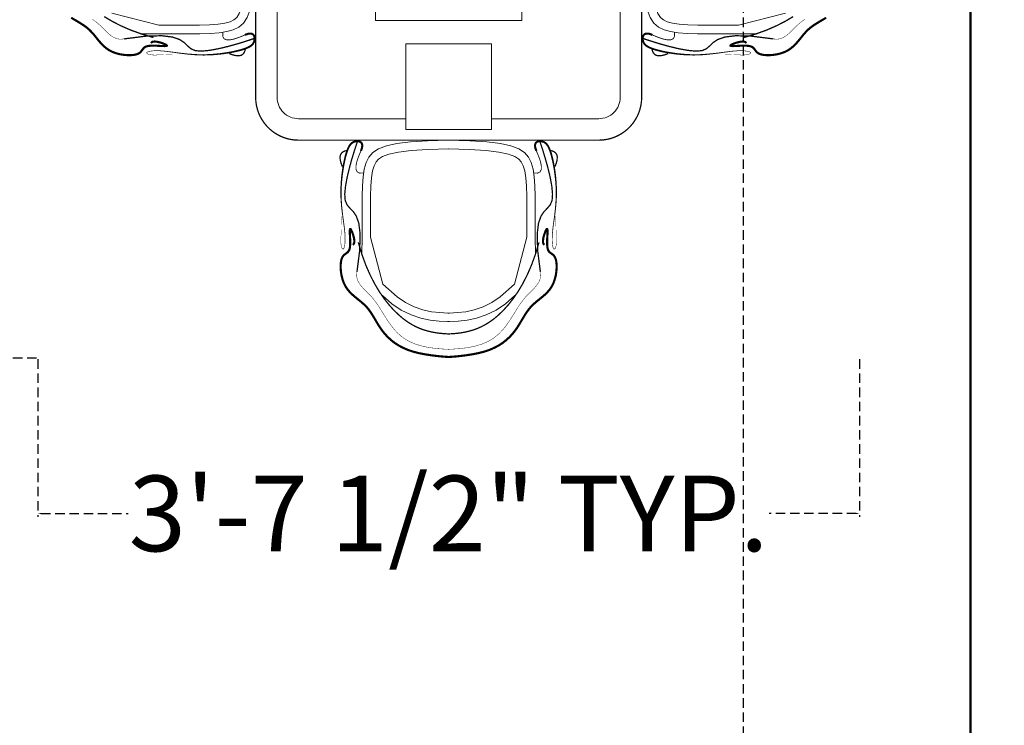
# Model space of a CAD drawing. Units: inches. Extents: x 513 to 1142, y 396 to 927.
# Tile 16 of 31: x 786 to 838, y 691 to 728. Entities that reach past the tile are written whole.
import ezdxf

# ---------------------------------------------------------------- set-up
doc = ezdxf.new("R2010")
doc.units = ezdxf.units.IN
doc.header["$MEASUREMENT"] = 0
doc.linetypes.add('DASHED', pattern=[0.75, 0.5, -0.25])
for name, color, linetype, lineweight in [('A-ANNO-DIMS', 2, 'DASHED', 18), ('A-WALL', 7, 'Continuous', 50), ('furniture', 92, 'Continuous', 18)]:
    doc.layers.add(name, color=color, linetype=linetype, lineweight=lineweight)
doc.styles.get("Standard").update_dxf_attribs({"font": 'arial.ttf'})
doc.dimstyles.get("Standard").update_dxf_attribs({"dimtxt": 4, "dimasz": 0.18, "dimexe": 0.18, "dimexo": 0.0625, "dimgap": 0.09, "dimtad": 0, "dimtih": 1, "dimtoh": 1, "dimdec": 0, "dimrnd": 6, "dimzin": 0, "dimdsep": 46, "dimlunit": 3, "dimtxsty": 'Standard', "dimcen": 0.09, "dimadec": 0, "dimazin": 0, "dimtfac": 1, "dimtdec": 0, "dimtofl": 0, "dimtmove": 0, "dimatfit": 3, "dimfxl": 1, "dimtolj": 1, "dimtzin": 0, "dimarcsym": 0})

# ---------------------------------------------------------------- blocks, each defined once
blk = doc.blocks.new('ОГ55_на6персон_стол1400х900')
for points, const_width in [([(-473.4, 523.4), (-471.2, 521.4), (-470.1, 518.2), (-469.9, 514.2), (-470.4, 509.6), (-471.4, 504.8), (-472.7, 500.1), (-474.2, 495.7), (-475.7, 492), (-477, 489.2), (-478, 487.3), (-478.9, 486.4), (-479.6, 486.4), (-480.1, 487.3), (-480.4, 489.1), (-480.6, 491.8), (-480.5, 495.4), (-480.3, 499.8), (-480, 504.9), (-479.7, 510.3), (-479.6, 516), (-479.6, 521.5), (-479.9, 526.8), (-480.6, 531.5), (-481.8, 535.5), (-483.5, 538.5), (-485.7, 540.8), (-488.2, 542.8), (-490.8, 544.6), (-493.4, 546.7), (-495.9, 549.3), (-498.1, 552.7), (-499.8, 557.2), (-501.1, 563.1), (-501.7, 570.2), (-501.7, 578.1), (-501, 586.6), (-499.6, 595.4), (-497.4, 604.2), (-494.3, 612.7), (-490.4, 620.6), (-485.5, 627.7), (-480, 634.2), (-473.9, 640.1), (-467.5, 645.6), (-460.9, 650.9), (-454.3, 656.2), (-448.1, 661.7), (-442.2, 667.5), (-436.9, 673.7), (-432.1, 680.3), (-427.6, 687.3), (-423.2, 694.5), (-418.9, 701.9), (-414.4, 709.4)], 5), ([(-463.8, 586.5), (-464.6, 595.2), (-463.4, 603), (-460.5, 610.1), (-456.3, 616.6), (-451.1, 622.8), (-445.3, 628.7), (-439.3, 634.6), (-433.4, 640.6), (-427.9, 646.8), (-422.8, 653.3), (-417.9, 659.9)], 1), ([(-460.6, 517.6), (-452.3, 545.4), (-443.2, 570.7), (-433.2, 593.6), (-422.7, 614.1), (-411.8, 632.4)], 3), ([(-463.8, 586.5), (-457.4, 535.5), (-456.4, 498.8), (-459.4, 473.4), (-465.3, 456.6), (-472.6, 445.7), (-480.2, 437.8), (-486.8, 430.2), (-491.2, 420), (-492.3, 405.3), (-490.5, 386.7), (-486.7, 366), (-481.6, 344.5), (-475.9, 323.8), (-470.3, 305.4), (-465.6, 291), (-462.5, 281.9)], 3), ([(-454.5, 304.2), (-457.8, 312), (-461.3, 321), (-464.3, 330.3), (-466.1, 339.3), (-466, 347.1), (-463.5, 353), (-457.8, 356.1), (-448.2, 355.7)], 2), ([(-498, 341), (-501.3, 331.8), (-503, 324.1), (-503.1, 317.8), (-501.9, 312.9), (-499.4, 309), (-495.8, 306.2), (-491.2, 304.3), (-485.7, 303.1)], 3), ([(-944.1, 52.8), (-942.1, 50.6), (-938.9, 49.4), (-934.9, 49.2), (-930.3, 49.7), (-925.5, 50.7), (-920.8, 52), (-916.4, 53.5), (-912.7, 55), (-909.9, 56.3), (-908, 57.4), (-907.1, 58.2), (-907.1, 58.9), (-908, 59.4), (-909.8, 59.7), (-912.5, 59.9), (-916.1, 59.8), (-920.5, 59.6), (-925.5, 59.3), (-931, 59), (-936.6, 58.9), (-942.2, 58.9), (-947.5, 59.2), (-952.2, 59.9), (-956.2, 61.1), (-959.2, 62.9), (-961.5, 65), (-963.4, 67.5), (-965.3, 70.1), (-967.4, 72.7), (-969.9, 75.2), (-973.4, 77.4), (-977.9, 79.2), (-983.8, 80.4), (-990.9, 81.1), (-998.8, 81.1), (-1007.3, 80.4), (-1016.1, 78.9), (-1024.9, 76.7), (-1033.4, 73.6), (-1041.3, 69.7), (-1048.4, 64.9), (-1054.8, 59.3), (-1060.7, 53.2), (-1066.3, 46.8), (-1071.6, 40.2), (-1076.9, 33.7), (-1082.4, 27.4), (-1088.1, 21.5), (-1094.4, 16.2), (-1101, 11.4), (-1108, 6.9), (-1115.2, 2.5), (-1122.6, -1.8), (-1130.1, -6.3), (-1137.6, -11.1), (-1145, -16.4), (-1152.3, -22.3), (-1159.4, -29), (-1166.2, -36.3), (-1172.7, -44.6), (-1178.7, -53.8), (-1184.1, -64), (-1189, -75.2), (-1193.2, -87.7), (-1196.7, -101.2), (-1199.4, -115.3), (-1201.6, -129.2), (-1203.2, -142.1), (-1204.4, -153.5), (-1205.1, -162.5), (-1205.5, -168.5), (-1205.7, -170.7)], 5), ([(-1007.2, 43.1), (-956.2, 36.7), (-919.4, 35.7), (-894.1, 38.7), (-877.3, 44.6), (-866.4, 51.9), (-858.5, 59.6), (-850.8, 66.2), (-840.7, 70.5), (-826, 71.6), (-807.4, 69.8), (-786.6, 66), (-765.2, 60.9), (-744.5, 55.2), (-726.1, 49.6), (-711.6, 44.9), (-702.6, 41.8)], 3), ([(-761.7, 77.3), (-752.5, 80.6), (-744.8, 82.3), (-738.5, 82.4), (-733.5, 81.2), (-729.7, 78.7), (-726.9, 75.1), (-725, 70.5), (-723.8, 65)], 3), ([(-724.9, 33.8), (-732.7, 37.2), (-741.6, 40.7), (-751, 43.6), (-760, 45.4), (-767.8, 45.4), (-773.6, 42.8), (-776.8, 37.1), (-776.4, 27.6)], 2), ([(-1007.2, 43.1), (-1015.9, 43.9), (-1023.6, 42.7), (-1030.7, 39.8), (-1037.3, 35.6), (-1043.5, 30.4), (-1049.4, 24.7), (-1055.3, 18.6), (-1061.3, 12.7), (-1067.5, 7.2), (-1073.9, 2.1), (-1080.6, -2.8), (-1087.4, -7.4), (-1094.3, -11.8), (-1101.4, -16.3), (-1108.5, -20.7), (-1115.7, -25.2), (-1122.9, -29.9), (-1130, -34.9), (-1137, -40.2), (-1143.8, -45.9), (-1150.3, -52.2), (-1156.4, -59), (-1162.1, -66.5), (-1167.3, -74.8), (-1171.9, -83.9), (-1175.9, -94), (-1179.3, -105.1), (-1182.2, -117.4), (-1184.5, -130.9), (-1186.2, -145.8), (-1187.4, -162.1), (-1187.8, -170.7)], 1), ([(-938.3, 40), (-966.1, 31.7), (-991.4, 22.5), (-1014.2, 12.5), (-1034.8, 2), (-1053.1, -8.9), (-1069.4, -20.1), (-1083.7, -31.3), (-1096.1, -42.5), (-1106.8, -53.5), (-1116, -64.2), (-1123.7, -74.7), (-1130.1, -84.9), (-1135.3, -94.9), (-1139.6, -104.7), (-1143, -114.3), (-1145.6, -123.7), (-1147.7, -132.7), (-1149.2, -141.4), (-1150.3, -149.3), (-1151, -156.4), (-1151.5, -162.3), (-1151.7, -166.8), (-1151.8, -169.6), (-1151.8, -170.7)], 3), ([(-944.1, -394.1), (-942.1, -391.9), (-938.9, -390.8), (-934.9, -390.6), (-930.3, -391.1), (-925.5, -392), (-920.8, -393.4), (-916.4, -394.9), (-912.7, -396.3), (-909.9, -397.6), (-908, -398.7), (-907.1, -399.6), (-907.1, -400.3), (-908, -400.8), (-909.8, -401.1), (-912.5, -401.2), (-916.1, -401.2), (-920.5, -401), (-925.5, -400.7), (-931, -400.4), (-936.6, -400.2), (-942.2, -400.3), (-947.5, -400.6), (-952.2, -401.3), (-956.2, -402.5), (-959.2, -404.2), (-961.5, -406.4), (-963.4, -408.8), (-965.3, -411.4), (-967.4, -414.1), (-969.9, -416.5), (-973.4, -418.7), (-977.9, -420.5), (-983.8, -421.8), (-990.9, -422.4), (-998.8, -422.4), (-1007.3, -421.7), (-1016.1, -420.3), (-1024.9, -418), (-1033.4, -415), (-1041.3, -411), (-1048.4, -406.2), (-1054.8, -400.7), (-1060.7, -394.6), (-1066.3, -388.1), (-1071.6, -381.6), (-1076.9, -375), (-1082.4, -368.7), (-1088.1, -362.9), (-1094.4, -357.6), (-1101, -352.8), (-1108, -348.2), (-1115.2, -343.9), (-1122.6, -339.5), (-1130.1, -335), (-1137.6, -330.2), (-1145, -324.9), (-1152.3, -319), (-1159.4, -312.4), (-1166.2, -305), (-1172.7, -296.8), (-1178.7, -287.6), (-1184.1, -277.4), (-1189, -266.1), (-1193.2, -253.7), (-1196.7, -240.1), (-1199.4, -226.1), (-1201.6, -212.2), (-1203.2, -199.2), (-1204.4, -187.9), (-1205.1, -178.9), (-1205.5, -172.9), (-1205.7, -170.7)], 5), ([(-1007.2, -384.5), (-1015.9, -385.3), (-1023.6, -384), (-1030.7, -381.1), (-1037.3, -376.9), (-1043.5, -371.8), (-1049.4, -366), (-1055.3, -360), (-1061.3, -354.1), (-1067.5, -348.6), (-1073.9, -343.4), (-1080.6, -338.6), (-1087.4, -334), (-1094.3, -329.5), (-1101.4, -325.1), (-1108.5, -320.7), (-1115.7, -316.1), (-1122.9, -311.4), (-1130, -306.5), (-1137, -301.2), (-1143.8, -295.4), (-1150.3, -289.2), (-1156.4, -282.3), (-1162.1, -274.8), (-1167.3, -266.5), (-1171.9, -257.4), (-1175.9, -247.3), (-1179.3, -236.2), (-1182.2, -224), (-1184.5, -210.5), (-1186.2, -195.6), (-1187.4, -179.3), (-1187.8, -170.7)], 1), ([(-938.3, -381.3), (-966.1, -373), (-991.4, -363.8), (-1014.2, -353.9), (-1034.8, -343.4), (-1053.1, -332.5), (-1069.4, -321.3), (-1083.7, -310), (-1096.1, -298.9), (-1106.8, -287.9), (-1116, -277.2), (-1123.7, -266.7), (-1130.1, -256.4), (-1135.3, -246.4), (-1139.6, -236.6), (-1143, -227), (-1145.6, -217.7), (-1147.7, -208.6), (-1149.2, -200), (-1150.3, -192), (-1151, -185), (-1151.5, -179.1), (-1151.7, -174.6), (-1151.8, -171.7), (-1151.8, -170.7)], 3), ([(-1007.2, -384.5), (-956.2, -378.1), (-919.4, -377.1), (-894.1, -380.1), (-877.3, -385.9), (-866.4, -393.3), (-858.5, -400.9), (-850.8, -407.5), (-840.7, -411.8), (-826, -412.9), (-807.4, -411.2), (-786.6, -407.4), (-765.2, -402.3), (-744.5, -396.5), (-726.1, -391), (-711.6, -386.3), (-702.6, -383.2)], 3), ([(-724.9, -375.1), (-732.7, -378.5), (-741.6, -382), (-751, -385), (-760, -386.8), (-767.8, -386.7), (-773.6, -384.2), (-776.8, -378.4), (-776.4, -368.9)], 2), ([(-761.7, -418.7), (-752.5, -422), (-744.8, -423.7), (-738.5, -423.8), (-733.5, -422.6), (-729.7, -420.1), (-726.9, -416.5), (-725, -411.9), (-723.8, -406.4)], 3), ([(-463.8, -927.9), (-457.4, -876.9), (-456.4, -840.1), (-459.4, -814.7), (-465.3, -798), (-472.6, -787), (-480.2, -779.2), (-486.8, -771.5), (-491.2, -761.4), (-492.3, -746.6), (-490.5, -728.1), (-486.7, -707.3), (-481.6, -685.8), (-475.9, -665.1), (-470.3, -646.8), (-465.6, -632.3), (-462.5, -623.2)], 3), ([(-498, -682.4), (-501.3, -673.2), (-503, -665.5), (-503.1, -659.2), (-501.9, -654.2), (-499.4, -650.4), (-495.8, -647.6), (-491.2, -645.6), (-485.7, -644.5)], 3), ([(-454.5, -645.6), (-457.8, -653.4), (-461.3, -662.3), (-464.3, -671.7), (-466.1, -680.7), (-466, -688.5), (-463.5, -694.3), (-457.8, -697.5), (-448.2, -697.1)], 2), ([(-473.4, -864.8), (-471.2, -862.7), (-470.1, -859.6), (-469.9, -855.5), (-470.4, -851), (-471.4, -846.2), (-472.7, -841.5), (-474.2, -837.1), (-475.7, -833.4), (-477, -830.6), (-478, -828.7), (-478.9, -827.8), (-479.6, -827.7), (-480.1, -828.6), (-480.4, -830.5), (-480.6, -833.2), (-480.5, -836.7), (-480.3, -841.2), (-480, -846.2), (-479.7, -851.7), (-479.6, -857.3), (-479.6, -862.9), (-479.9, -868.2), (-480.6, -872.9), (-481.8, -876.8), (-483.5, -879.9), (-485.7, -882.2), (-488.2, -884.1), (-490.8, -886), (-493.4, -888), (-495.9, -890.6), (-498.1, -894), (-499.8, -898.6), (-501.1, -904.5), (-501.7, -911.6), (-501.7, -919.5), (-501, -928), (-499.6, -936.8), (-497.4, -945.6), (-494.3, -954.1), (-490.4, -962), (-485.5, -969.1), (-480, -975.5), (-473.9, -981.4), (-467.5, -986.9), (-460.9, -992.3), (-454.3, -997.6), (-448.1, -1003), (-442.2, -1008.8), (-436.9, -1015.1), (-432.1, -1021.7), (-427.6, -1028.7), (-423.2, -1035.9), (-418.9, -1043.3), (-414.4, -1050.8)], 5), ([(-460.6, -859), (-452.3, -886.8), (-443.2, -912.1), (-433.2, -934.9), (-422.7, -955.5), (-411.8, -973.8)], 3), ([(-463.8, -927.9), (-464.6, -936.5), (-463.4, -944.3), (-460.5, -951.4), (-456.3, -958), (-451.1, -964.1), (-445.3, -970.1), (-439.3, -976), (-433.4, -982), (-427.9, -988.2), (-422.8, -994.6), (-417.9, -1001.3)], 1)]:
    blk.add_lwpolyline(points, dxfattribs=dict(const_width=const_width))
for points in [[(-403.6, 615), (-431.9, 505.2), (-431.9, 469.2), (-432, 437.6), (-431.9, 410.1), (-431.2, 386.6), (-429.8, 367), (-427.3, 351.1), (-423.8, 338.8), (-419.4, 329.9), (-413.6, 323.3), (-404.4, 317.4), (-389.5, 311.8), (-367.3, 307), (-337.1, 303.4), (-298.1, 300.9), (-249.4, 299.3)], [(-452.3, 545.4), (-451.9, 505.1), (-451.9, 469.2), (-452, 437.5), (-451.9, 409.8), (-451.2, 385.6), (-449.6, 364.7), (-446.8, 346.8), (-442.5, 331.5), (-436.1, 318.7), (-426.8, 308), (-413.5, 299.4), (-395.1, 292.5), (-370.6, 287.3), (-339, 283.5), (-299.1, 280.9), (-250, 279.3)], [(-966.1, 31.7), (-925.8, 31.2), (-889.9, 31.2), (-858.2, 31.3), (-830.4, 31.2), (-806.3, 30.5), (-785.4, 29), (-767.4, 26.2), (-752.2, 21.8), (-739.4, 15.4), (-728.7, 6.1), (-720.1, -7.2), (-713.2, -25.6), (-708, -50.1), (-704.2, -81.7), (-701.6, -121.6), (-700, -170.7)], [(-1035.7, -17.1), (-925.9, 11.2), (-889.9, 11.2), (-858.2, 11.3), (-830.8, 11.2), (-807.3, 10.5), (-787.6, 9.1), (-771.7, 6.6), (-759.5, 3.1), (-750.6, -1.3), (-744, -7.1), (-738, -16.3), (-732.5, -31.2), (-727.7, -53.4), (-724.1, -83.6), (-721.5, -122.5), (-720, -171.3)], [(-1062.3, -16.7), (-1081.4, -38.1), (-1096.2, -60.3), (-1107.2, -82.9), (-1114.8, -105.5), (-1119.7, -127.5), (-1122.3, -148.6), (-1123.1, -168.3), (-1123.1, -170.7)], [(-1035.7, -17.1), (-1065.6, -50.4), (-1078.8, -70.2), (-1088.7, -90.5), (-1095.5, -110.8), (-1100, -130.9), (-1102.3, -150.3), (-1103.1, -168.6), (-1103.1, -170.3)], [(-1062.3, -324.6), (-1081.4, -303.3), (-1096.2, -281.1), (-1107.2, -258.5), (-1114.8, -235.9), (-1119.7, -213.8), (-1122.3, -192.7), (-1123.1, -173), (-1123.1, -170.7)], [(-1035.7, -324.3), (-1065.6, -291), (-1078.8, -271.1), (-1088.7, -250.9), (-1095.5, -230.5), (-1100, -210.5), (-1102.3, -191.1), (-1103.1, -172.8), (-1103.1, -171.1)], [(-1035.7, -324.3), (-925.9, -352.6), (-889.9, -352.6), (-858.2, -352.7), (-830.8, -352.6), (-807.3, -351.9), (-787.6, -350.4), (-771.7, -348), (-759.5, -344.4), (-750.6, -340), (-744, -334.2), (-738, -325.1), (-732.5, -310.2), (-727.7, -288), (-724.1, -257.8), (-721.5, -218.8), (-720, -170)], [(-966.1, -373), (-925.8, -372.6), (-889.9, -372.6), (-858.2, -372.7), (-830.4, -372.6), (-806.3, -371.9), (-785.4, -370.3), (-767.4, -367.5), (-752.2, -363.2), (-739.4, -356.8), (-728.7, -347.5), (-720.1, -334.1), (-713.2, -315.8), (-708, -291.3), (-704.2, -259.6), (-701.6, -219.8), (-700, -170.7)], [(-452.3, -886.8), (-451.9, -846.4), (-451.9, -810.6), (-452, -778.9), (-451.9, -751.1), (-451.2, -726.9), (-449.6, -706), (-446.8, -688.1), (-442.5, -672.9), (-436.1, -660), (-426.8, -649.4), (-413.5, -640.7), (-395.1, -633.9), (-370.6, -628.7), (-339, -624.8), (-299.1, -622.2), (-250, -620.7)], [(-403.6, -956.4), (-431.9, -846.6), (-431.9, -810.5), (-432, -778.9), (-431.9, -751.4), (-431.2, -728), (-429.8, -708.3), (-427.3, -692.4), (-423.8, -680.1), (-419.4, -671.3), (-413.6, -664.7), (-404.4, -658.7), (-389.5, -653.1), (-367.3, -648.4), (-337.1, -644.8), (-298.1, -642.2), (-249.4, -640.7)]]:
    blk.add_lwpolyline(points)
for points, format in [([(-454.5, 304.2, 5, 4.91, 0), (-452, 297.4, 4.91, 4.84, 0), (-451.3, 292.1, 4.84, 4.78, 0), (-451.9, 288.1, 4.78, 4.74, 0), (-453.7, 285.1, 4.74, 4.7, 0), (-456.3, 283.2, 4.7, 4.65, 0), (-459.4, 282.2, 4.65, 4.61, 0), (-462.9, 281.8, 4.61, 4.56, 0), (-466.5, 282.1, 4.56, 4.52, 0), (-469.8, 282.8, 4.52, 4.47, 0), (-472.9, 284.1, 4.47, 4.43, 0), (-475.9, 286.1, 4.43, 4.38, 0), (-478.7, 288.8, 4.38, 4.32, 0), (-481.3, 292.5, 4.32, 4.25, 0), (-483.8, 297.3, 4.25, 4.17, 0), (-486.3, 303.2, 4.17, 4.07, 0), (-488.7, 310.4, 4.07, 3.95, 0), (-491, 318.9, 3.95, 3.82, 0), (-493.3, 328.7, 3.82, 3.68, 0), (-495.4, 339.4, 3.68, 3.53, 0), (-497.2, 350.9, 3.53, 3.37, 0), (-498.8, 363, 3.37, 3.21, 0), (-500, 375.5, 3.21, 3.05, 0), (-500.8, 388.2, 3.05, 2.88, 0), (-501.1, 400.7, 2.88, 2.72, 0), (-500.9, 413.1, 2.72, 2.57, 0), (-500.2, 425.1, 2.57, 2.41, 0), (-499.2, 436.7, 2.41, 2.27, 0), (-498, 447.8, 2.27, 2.13, 0), (-496.7, 458.3, 2.13, 2, 0), (-495.3, 468.2, 2, 1.88, 0), (-494.1, 477.3, 1.88, 1.78, 0), (-493, 485.6, 1.78, 1.68, 0), (-492.2, 493.1, 1.68, 1.59, 0), (-491.7, 499.6, 1.59, 1.52, 0), (-491.4, 505.4, 1.52, 1.45, 0), (-491.3, 510.5, 1.45, 1.4, 0), (-491.4, 514.9, 1.4, 1.35, 0), (-491.6, 518.7, 1.35, 1.3, 0), (-492, 521.9, 1.3, 1.27, 0), (-492.4, 524.7, 1.27, 1.24, 0), (-492.8, 527, 1.24, 1.21, 0), (-493.3, 528.8, 1.21, 1.19, 0), (-493.8, 530.3, 1.19, 1.18, 0), (-494.3, 531.5, 1.18, 1.16, 0), (-494.8, 532.3, 1.16, 1.15, 0), (-495.3, 532.9, 1.15, 1.14, 0), (-495.8, 533.2, 1.14, 1.14, 0), (-496.3, 533.3, 1.14, 1.13, 0), (-496.8, 533.2, 1.13, 1.12, 0), (-497.3, 533, 1.12, 1.12, 0), (-497.8, 532.5, 1.12, 1.11, 0), (-498.3, 531.9, 1.11, 1.09, 0), (-498.7, 531.1, 1.09, 1.08, 0), (-499.1, 530.2, 1.08, 1.07, 0), (-499.5, 529.1, 1.07, 1.05, 0), (-499.9, 527.9, 1.05, 1.03, 0), (-500.3, 526.5, 1.03, 1.01, 0), (-500.6, 524.9, 1.01, 0.986, 0), (-500.9, 523.1, 0.986, 0.959, 0), (-501.1, 521, 0.959, 0.926, 0), (-501.3, 518.5, 0.926, 0.889, 0), (-501.4, 515.7, 0.889, 0.846, 0), (-501.4, 512.3, 0.846, 0.796, 0), (-501.3, 508.5, 0.796, 0.738, 0), (-501.1, 504, 0.738, 0.672, 0), (-500.8, 498.9, 0.672, 0.595, 0), (-500.6, 493, 0.595, 0.506, 0), (-500.3, 486.1, 0.506, 0.404, 0), (-500.1, 478.2, 0.404, 0.286, 0), (-499.9, 469.2, 0.286, 0.152, 0), (-499.9, 458.8, 0.152, 0, 0), (-500, 447.1, 0, 0, 0)], "xyseb"), ([(-650, -70.7), (-650, 179.3, -0.414214), (-600, 229.3), (-350, 229.3)], "xyb"), ([(-724.9, 33.8, 5, 4.91, 0), (-718.1, 31.4, 4.91, 4.84, 0), (-712.8, 30.6, 4.84, 4.78, 0), (-708.7, 31.2, 4.78, 4.74, 0), (-705.8, 33, 4.74, 4.7, 0), (-703.9, 35.6, 4.7, 4.65, 0), (-702.9, 38.8, 4.65, 4.61, 0), (-702.5, 42.3, 4.61, 4.56, 0), (-702.8, 45.8, 4.56, 4.52, 0), (-703.5, 49.1, 4.52, 4.47, 0), (-704.8, 52.2, 4.47, 4.43, 0), (-706.7, 55.2, 4.43, 4.38, 0), (-709.5, 58, 4.38, 4.32, 0), (-713.2, 60.6, 4.32, 4.25, 0), (-717.9, 63.2, 4.25, 4.17, 0), (-723.8, 65.6, 4.17, 4.07, 0), (-731, 68, 4.07, 3.95, 0), (-739.6, 70.4, 3.95, 3.82, 0), (-749.3, 72.6, 3.82, 3.68, 0), (-760.1, 74.7, 3.68, 3.53, 0), (-771.6, 76.5, 3.53, 3.37, 0), (-783.7, 78.1, 3.37, 3.21, 0), (-796.2, 79.3, 3.21, 3.05, 0), (-808.8, 80.1, 3.05, 2.88, 0), (-821.4, 80.4, 2.88, 2.72, 0), (-833.8, 80.2, 2.72, 2.57, 0), (-845.8, 79.5, 2.57, 2.41, 0), (-857.4, 78.6, 2.41, 2.27, 0), (-868.5, 77.3, 2.27, 2.13, 0), (-879, 76, 2.13, 2, 0), (-888.9, 74.6, 2, 1.88, 0), (-898, 73.4, 1.88, 1.78, 0), (-906.3, 72.3, 1.78, 1.68, 0), (-913.7, 71.5, 1.68, 1.59, 0), (-920.3, 71, 1.59, 1.52, 0), (-926.1, 70.7, 1.52, 1.45, 0), (-931.2, 70.7, 1.45, 1.4, 0), (-935.6, 70.7, 1.4, 1.35, 0), (-939.4, 71, 1.35, 1.3, 0), (-942.6, 71.3, 1.3, 1.27, 0), (-945.3, 71.7, 1.27, 1.24, 0), (-947.6, 72.1, 1.24, 1.21, 0), (-949.5, 72.6, 1.21, 1.19, 0), (-951, 73.1, 1.19, 1.18, 0), (-952.2, 73.6, 1.18, 1.16, 0), (-953, 74.1, 1.16, 1.15, 0), (-953.6, 74.6, 1.15, 1.14, 0), (-953.9, 75.1, 1.14, 1.14, 0), (-954, 75.6, 1.14, 1.13, 0), (-953.9, 76.2, 1.13, 1.12, 0), (-953.6, 76.6, 1.12, 1.12, 0), (-953.2, 77.1, 1.12, 1.11, 0), (-952.6, 77.6, 1.11, 1.09, 0), (-951.8, 78, 1.09, 1.08, 0), (-950.9, 78.4, 1.08, 1.07, 0), (-949.8, 78.9, 1.07, 1.05, 0), (-948.6, 79.2, 1.05, 1.03, 0), (-947.2, 79.6, 1.03, 1.01, 0), (-945.6, 79.9, 1.01, 0.986, 0), (-943.8, 80.2, 0.986, 0.959, 0), (-941.7, 80.4, 0.959, 0.926, 0), (-939.2, 80.6, 0.926, 0.889, 0), (-936.3, 80.7, 0.889, 0.846, 0), (-933, 80.7, 0.846, 0.796, 0), (-929.1, 80.6, 0.796, 0.738, 0), (-924.7, 80.4, 0.738, 0.672, 0), (-919.6, 80.2, 0.672, 0.595, 0), (-913.7, 79.9, 0.595, 0.506, 0), (-906.8, 79.6, 0.506, 0.404, 0), (-898.9, 79.4, 0.404, 0.286, 0), (-889.9, 79.2, 0.286, 0.152, 0), (-879.5, 79.2, 0.152, 0, 0), (-867.8, 79.4, 0, 0, 0)], "xyseb"), ([(-350, -570.7), (-600, -570.7, -0.414214), (-650, -520.7), (-650, -270.7)], "xyb"), ([(-724.9, -375.1, 5, 4.91, 0), (-718.1, -372.7, 4.91, 4.84, 0), (-712.8, -372, 4.84, 4.78, 0), (-708.7, -372.6, 4.78, 4.74, 0), (-705.8, -374.3, 4.74, 4.7, 0), (-703.9, -376.9, 4.7, 4.65, 0), (-702.9, -380.1, 4.65, 4.61, 0), (-702.5, -383.6, 4.61, 4.56, 0), (-702.8, -387.1, 4.56, 4.52, 0), (-703.5, -390.5, 4.52, 4.47, 0), (-704.8, -393.6, 4.47, 4.43, 0), (-706.7, -396.6, 4.43, 4.38, 0), (-709.5, -399.3, 4.38, 4.32, 0), (-713.2, -402, 4.32, 4.25, 0), (-717.9, -404.5, 4.25, 4.17, 0), (-723.8, -407, 4.17, 4.07, 0), (-731, -409.4, 4.07, 3.95, 0), (-739.6, -411.7, 3.95, 3.82, 0), (-749.3, -414, 3.82, 3.68, 0), (-760.1, -416, 3.68, 3.53, 0), (-771.6, -417.9, 3.53, 3.37, 0), (-783.7, -419.5, 3.37, 3.21, 0), (-796.2, -420.7, 3.21, 3.05, 0), (-808.8, -421.5, 3.05, 2.88, 0), (-821.4, -421.8, 2.88, 2.72, 0), (-833.8, -421.6, 2.72, 2.57, 0), (-845.8, -420.9, 2.57, 2.41, 0), (-857.4, -419.9, 2.41, 2.27, 0), (-868.5, -418.7, 2.27, 2.13, 0), (-879, -417.4, 2.13, 2, 0), (-888.9, -416, 2, 1.88, 0), (-898, -414.7, 1.88, 1.78, 0), (-906.3, -413.7, 1.78, 1.68, 0), (-913.7, -412.9, 1.68, 1.59, 0), (-920.3, -412.4, 1.59, 1.52, 0), (-926.1, -412.1, 1.52, 1.45, 0), (-931.2, -412, 1.45, 1.4, 0), (-935.6, -412.1, 1.4, 1.35, 0), (-939.4, -412.3, 1.35, 1.3, 0), (-942.6, -412.7, 1.3, 1.27, 0), (-945.3, -413, 1.27, 1.24, 0), (-947.6, -413.5, 1.24, 1.21, 0), (-949.5, -413.9, 1.21, 1.19, 0), (-951, -414.4, 1.19, 1.18, 0), (-952.2, -414.9, 1.18, 1.16, 0), (-953, -415.4, 1.16, 1.15, 0), (-953.6, -416, 1.15, 1.14, 0), (-953.9, -416.5, 1.14, 1.14, 0), (-954, -417, 1.14, 1.13, 0), (-953.9, -417.5, 1.13, 1.12, 0), (-953.6, -418, 1.12, 1.12, 0), (-953.2, -418.5, 1.12, 1.11, 0), (-952.6, -418.9, 1.11, 1.09, 0), (-951.8, -419.4, 1.09, 1.08, 0), (-950.9, -419.8, 1.08, 1.07, 0), (-949.8, -420.2, 1.07, 1.05, 0), (-948.6, -420.6, 1.05, 1.03, 0), (-947.2, -421, 1.03, 1.01, 0), (-945.6, -421.3, 1.01, 0.986, 0), (-943.8, -421.6, 0.986, 0.959, 0), (-941.7, -421.8, 0.959, 0.926, 0), (-939.2, -422, 0.926, 0.889, 0), (-936.3, -422, 0.889, 0.846, 0), (-933, -422, 0.846, 0.796, 0), (-929.1, -422, 0.796, 0.738, 0), (-924.7, -421.8, 0.738, 0.672, 0), (-919.6, -421.5, 0.672, 0.595, 0), (-913.7, -421.2, 0.595, 0.506, 0), (-906.8, -421, 0.506, 0.404, 0), (-898.9, -420.7, 0.404, 0.286, 0), (-889.9, -420.6, 0.286, 0.152, 0), (-879.5, -420.6, 0.152, 0, 0), (-867.8, -420.7, 0, 0, 0)], "xyseb"), ([(-454.5, -645.6, 5, 4.91, 0), (-452, -638.8, 4.91, 4.84, 0), (-451.3, -633.5, 4.84, 4.78, 0), (-451.9, -629.4, 4.78, 4.74, 0), (-453.7, -626.5, 4.74, 4.7, 0), (-456.3, -624.6, 4.7, 4.65, 0), (-459.4, -623.5, 4.65, 4.61, 0), (-462.9, -623.2, 4.61, 4.56, 0), (-466.5, -623.5, 4.56, 4.52, 0), (-469.8, -624.2, 4.52, 4.47, 0), (-472.9, -625.5, 4.47, 4.43, 0), (-475.9, -627.4, 4.43, 4.38, 0), (-478.7, -630.2, 4.38, 4.32, 0), (-481.3, -633.9, 4.32, 4.25, 0), (-483.8, -638.6, 4.25, 4.17, 0), (-486.3, -644.5, 4.17, 4.07, 0), (-488.7, -651.7, 4.07, 3.95, 0), (-491, -660.3, 3.95, 3.82, 0), (-493.3, -670, 3.82, 3.68, 0), (-495.4, -680.8, 3.68, 3.53, 0), (-497.2, -692.3, 3.53, 3.37, 0), (-498.8, -704.4, 3.37, 3.21, 0), (-500, -716.9, 3.21, 3.05, 0), (-500.8, -729.5, 3.05, 2.88, 0), (-501.1, -742.1, 2.88, 2.72, 0), (-500.9, -754.5, 2.72, 2.57, 0), (-500.2, -766.5, 2.57, 2.41, 0), (-499.2, -778.1, 2.41, 2.27, 0), (-498, -789.2, 2.27, 2.13, 0), (-496.7, -799.7, 2.13, 2, 0), (-495.3, -809.6, 2, 1.88, 0), (-494.1, -818.7, 1.88, 1.78, 0), (-493, -827, 1.78, 1.68, 0), (-492.2, -834.4, 1.68, 1.59, 0), (-491.7, -841, 1.59, 1.52, 0), (-491.4, -846.8, 1.52, 1.45, 0), (-491.3, -851.9, 1.45, 1.4, 0), (-491.4, -856.3, 1.4, 1.35, 0), (-491.6, -860.1, 1.35, 1.3, 0), (-492, -863.3, 1.3, 1.27, 0), (-492.4, -866, 1.27, 1.24, 0), (-492.8, -868.3, 1.24, 1.21, 0), (-493.3, -870.2, 1.21, 1.19, 0), (-493.8, -871.7, 1.19, 1.18, 0), (-494.3, -872.9, 1.18, 1.16, 0), (-494.8, -873.7, 1.16, 1.15, 0), (-495.3, -874.3, 1.15, 1.14, 0), (-495.8, -874.6, 1.14, 1.14, 0), (-496.3, -874.7, 1.14, 1.13, 0), (-496.8, -874.6, 1.13, 1.12, 0), (-497.3, -874.3, 1.12, 1.12, 0), (-497.8, -873.9, 1.12, 1.11, 0), (-498.3, -873.3, 1.11, 1.09, 0), (-498.7, -872.5, 1.09, 1.08, 0), (-499.1, -871.6, 1.08, 1.07, 0), (-499.5, -870.5, 1.07, 1.05, 0), (-499.9, -869.2, 1.05, 1.03, 0), (-500.3, -867.9, 1.03, 1.01, 0), (-500.6, -866.3, 1.01, 0.986, 0), (-500.9, -864.5, 0.986, 0.959, 0), (-501.1, -862.4, 0.959, 0.926, 0), (-501.3, -859.9, 0.926, 0.889, 0), (-501.4, -857, 0.889, 0.846, 0), (-501.4, -853.7, 0.846, 0.796, 0), (-501.3, -849.8, 0.796, 0.738, 0), (-501.1, -845.4, 0.738, 0.672, 0), (-500.8, -840.3, 0.672, 0.595, 0), (-500.6, -834.3, 0.595, 0.506, 0), (-500.3, -827.5, 0.506, 0.404, 0), (-500.1, -819.6, 0.404, 0.286, 0), (-499.9, -810.5, 0.286, 0.152, 0), (-499.9, -800.2, 0.152, 0, 0), (-500, -788.5, 0, 0, 0)], "xyseb")]:
    blk.add_lwpolyline(points, format=format)
at = {"const_width": 3}
blk.add_lwpolyline([(-600, 279.3), (600, 279.3, -0.414214), (700, 179.3), (700, -520.7, -0.414214), (600, -620.7), (-600, -620.7, -0.414214), (-700, -520.7), (-700, 179.3, -0.414214)], format="xyb", close=True, dxfattribs=at)
for points in [[(-420.7, -341.4), (420.7, -341.4), (420.7, 0), (-420.7, 0)], [(-675, -270.7), (-475, -270.7), (-475, -70.7), (-675, -70.7)]]:
    blk.add_lwpolyline(points, close=True)
blk = doc.blocks.new('*D121')
at = {"layer": 'A-ANNO-DIMS', "color": 0, "lineweight": -2, "transparency": 16777216}
for p, q in [((786.62, 765.256), (778.284, 765.256)), ((778.464, 765.076), (778.464, 740.017)), ((778.464, 710.643), (778.464, 735.701)), ((786.62, 710.463), (778.284, 710.463))]:
    blk.add_line(p, q, dxfattribs=at)
at = {"layer": 'A-ANNO-DIMS', "color": 0, "transparency": 16777216}
for points in [[(778.434, 765.076), (778.494, 765.076), (778.464, 765.256)], [(778.434, 710.643), (778.494, 710.643), (778.464, 710.463)]]:
    blk.add_solid(points, dxfattribs=at)
at = {"layer": 'Defpoints', "color": 0, "transparency": 16777216}
for p in [(778.464, 765.256), (786.683, 765.256), (786.683, 710.463)]:
    blk.add_point(p, dxfattribs=at)
at = {"layer": 'A-ANNO-DIMS', "color": 0, "transparency": 16777216, "insert": (778.464, 737.859), "char_height": 4, "attachment_point": 5}
blk.add_mtext('\\A1;DINING SET 4\'-7" TYP.', dxfattribs=at)
blk = doc.blocks.new('*D122')
at = {"layer": 'A-ANNO-DIMS', "color": 0, "lineweight": -2, "transparency": 16777216}
for p, q in [((786.683, 710.4), (786.683, 702.064)), ((830.138, 710.4), (830.138, 702.064)), ((786.863, 702.244), (791.47, 702.244)), ((829.958, 702.244), (825.35, 702.244))]:
    blk.add_line(p, q, dxfattribs=at)
at = {"layer": 'A-ANNO-DIMS', "color": 0, "transparency": 16777216}
for points in [[(786.863, 702.274), (786.863, 702.214), (786.683, 702.244)], [(829.958, 702.274), (829.958, 702.214), (830.138, 702.244)]]:
    blk.add_solid(points, dxfattribs=at)
at = {"layer": 'Defpoints', "color": 0, "transparency": 16777216}
for p in [(786.683, 710.463), (830.138, 710.463), (786.683, 702.244)]:
    blk.add_point(p, dxfattribs=at)
at = {"layer": 'A-ANNO-DIMS', "color": 0, "transparency": 16777216, "insert": (808.41, 702.244), "char_height": 4, "attachment_point": 5}
blk.add_mtext('\\A1;3\'-7 1/2" TYP.', dxfattribs=at)
blk = doc.blocks.new('*D136')
at = {"layer": 'A-ANNO-DIMS', "color": 0, "lineweight": -2, "transparency": 16777216}
for p, q in [((835.995, 770.096), (835.995, 401.578)), ((743.802, 768.607), (743.802, 401.578)), ((743.982, 401.758), (784.509, 401.758)), ((835.815, 401.758), (795.289, 401.758))]:
    blk.add_line(p, q, dxfattribs=at)
at = {"layer": 'A-ANNO-DIMS', "color": 0, "transparency": 16777216}
for points in [[(743.982, 401.788), (743.982, 401.728), (743.802, 401.758)], [(835.815, 401.788), (835.815, 401.728), (835.995, 401.758)]]:
    blk.add_solid(points, dxfattribs=at)
at = {"layer": 'Defpoints', "color": 0, "transparency": 16777216}
for p in [(835.995, 770.158), (743.802, 768.67), (835.995, 401.758)]:
    blk.add_point(p, dxfattribs=at)
at = {"layer": 'A-ANNO-DIMS', "color": 0, "transparency": 16777216, "insert": (789.899, 401.758), "char_height": 4, "attachment_point": 5}
blk.add_mtext('\\A1;7\'-8"', dxfattribs=at)
blk = doc.blocks.new('*D169')
at = {"layer": 'A-ANNO-DIMS', "color": 0, "lineweight": -2, "transparency": 16777216}
for p, q in [((835.995, 774.096), (835.995, 401.578)), ((839.995, 774.096), (839.995, 401.578)), ((836.175, 401.758), (839.815, 401.758)), ((839.995, 401.758), (840.175, 401.758))]:
    blk.add_line(p, q, dxfattribs=at)
at = {"layer": 'A-ANNO-DIMS', "color": 0, "transparency": 16777216}
for points in [[(836.175, 401.788), (836.175, 401.728), (835.995, 401.758)], [(839.815, 401.788), (839.815, 401.728), (839.995, 401.758)]]:
    blk.add_solid(points, dxfattribs=at)
at = {"layer": 'Defpoints', "color": 0, "transparency": 16777216}
for p in [(835.995, 774.158), (839.995, 774.158), (839.995, 401.758)]:
    blk.add_point(p, dxfattribs=at)
at = {"layer": 'A-ANNO-DIMS', "color": 0, "transparency": 16777216, "insert": (845.582, 401.758), "char_height": 4, "attachment_point": 5}
blk.add_mtext('\\A1;0\'-4"', dxfattribs=at)
blk = doc.blocks.new('*D175')
at = {"layer": 'A-ANNO-DIMS', "color": 0, "lineweight": -2, "transparency": 16777216}
for p, q in [((772.995, 637.221), (772.995, 920.738)), ((773.175, 920.558), (793.008, 920.558)), ((823.815, 920.558), (803.982, 920.558)), ((823.995, 637.221), (823.995, 920.738))]:
    blk.add_line(p, q, dxfattribs=at)
at = {"layer": 'A-ANNO-DIMS', "color": 0, "transparency": 16777216}
for points in [[(773.175, 920.588), (773.175, 920.528), (772.995, 920.558)], [(823.815, 920.588), (823.815, 920.528), (823.995, 920.558)]]:
    blk.add_solid(points, dxfattribs=at)
at = {"layer": 'Defpoints', "color": 0, "transparency": 16777216}
for p in [(823.995, 920.558), (772.995, 637.158), (823.995, 637.158)]:
    blk.add_point(p, dxfattribs=at)
at = {"layer": 'A-ANNO-DIMS', "color": 0, "transparency": 16777216, "insert": (798.495, 920.558), "char_height": 4, "attachment_point": 5}
blk.add_mtext('\\A1;4\'-3"', dxfattribs=at)

msp = doc.modelspace()

# ---------------------------------------------------------------- linework, layer by layer
at = {"layer": 'A-WALL'}
msp.add_line((835.995, 770.158), (835.995, 641.158), dxfattribs=at)

# ---------------------------------------------------------------- block references
at = {"layer": 'furniture', "xscale": 0.022676467704094, "yscale": 0.022676467704094, "zscale": 0.022676467704094, "rotation": 90}
msp.add_blockref('ОГ55_на6персон_стол1400х900', (804.54, 737.859), dxfattribs=at)

# ---------------------------------------------------------------- dimensions: what is measured, and where the dimension line sits
at = {"layer": 'A-ANNO-DIMS'}
for base, p1, p2, picture, middle in [((823.995, 920.558), (772.995, 637.158), (823.995, 637.158), '*D175', (798.495, 920.558)), ((839.995, 401.758), (835.995, 774.158), (839.995, 774.158), '*D169', (845.582, 401.758)), ((835.995, 401.758), (743.802, 768.67), (835.995, 770.158), '*D136', (789.899, 401.758))]:
    dim = msp.add_linear_dim(base=base, p1=p1, p2=p2, dimstyle='Standard', override={"dimdec": 1, "dimlfac": 1, "dimrnd": 0, "dimzin": 1, "dimdsep": 46, "dimlunit": 4, "dimfrac": 2}, dxfattribs=at)
    dim.commit()
    dim.dimension.update_dxf_attribs({"geometry": picture, "text_midpoint": middle})
for base, p1, p2, angle, text, picture, middle in [((778.464, 765.256), (786.683, 710.463), (786.683, 765.256), 90, 'DINING SET <> TYP.', '*D121', (778.464, 737.859)), ((786.683, 702.244), (830.138, 710.463), (786.683, 710.463), 180, '<> TYP.', '*D122', (808.41, 702.244))]:
    dim = msp.add_linear_dim(base=base, p1=p1, p2=p2, angle=angle, text=text, dimstyle='Standard', override={"dimdec": 1, "dimlfac": 1, "dimrnd": 0, "dimzin": 1, "dimdsep": 46, "dimlunit": 4, "dimfrac": 2}, dxfattribs=at)
    dim.commit()
    dim.dimension.update_dxf_attribs({"geometry": picture, "text_midpoint": middle})

doc.saveas('drawing.dxf')
